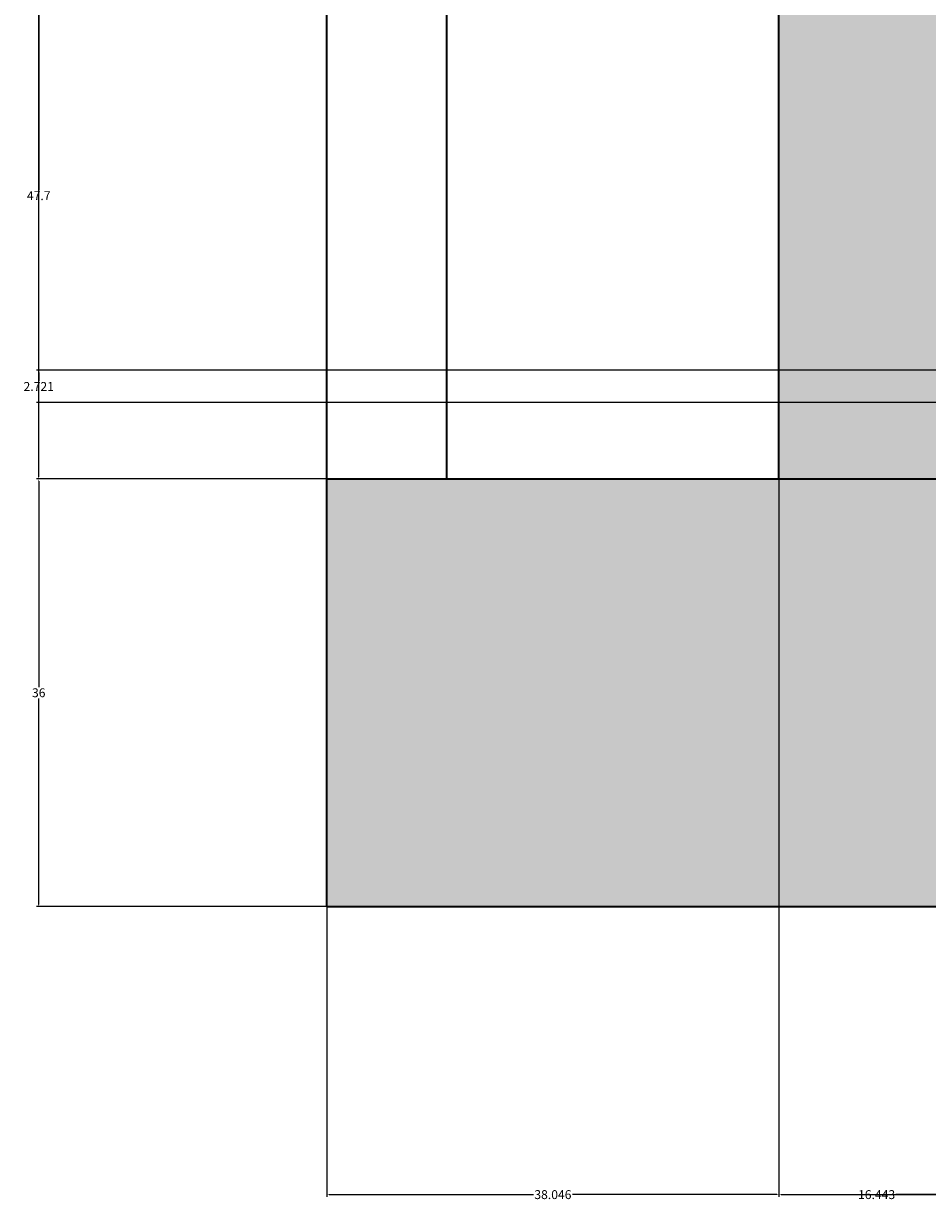
# Model space of a CAD drawing. Units: inches. Extents: x 62 to 566, y 66 to 528.
# Tile 1 of 20: x 62 to 138, y 66 to 165. Entities that reach past the tile are written whole.
import ezdxf

# ---------------------------------------------------------------- set-up
doc = ezdxf.new("R2010")
doc.units = ezdxf.units.IN
doc.header["$MEASUREMENT"] = 0
for name, color, linetype, lineweight in [('A-ANNO-DIMS', 2, 'Continuous', 18), ('A-ELEV', 7, 'Continuous', 35), ('A-WALL-PATT', 8, 'Continuous', 13)]:
    doc.layers.add(name, color=color, linetype=linetype, lineweight=lineweight)
doc.styles.get("Standard").update_dxf_attribs({"font": 'arial.ttf'})
doc.dimstyles.get("Standard").update_dxf_attribs({"dimtxt": 0.75, "dimasz": 0.18, "dimexe": 0.18, "dimexo": 0.0625, "dimgap": 0.09, "dimtad": 0, "dimtih": 1, "dimtoh": 1, "dimdec": 4, "dimzin": 0, "dimdsep": 46, "dimlunit": 4, "dimtxsty": 'Standard', "dimcen": 0.09, "dimadec": 0, "dimazin": 0, "dimtfac": 1, "dimtdec": 4, "dimtofl": 0, "dimtmove": 0, "dimatfit": 3, "dimfxl": 1, "dimtolj": 1, "dimtzin": 0, "dimarcsym": 0})

# ---------------------------------------------------------------- blocks, each defined once
blk = doc.blocks.new('*D7')
at = {"layer": 'A-ANNO-DIMS', "color": 0, "lineweight": -2, "transparency": 16777216}
for p, q in [((125.942, 126.306), (125.942, 65.939)), ((87.896, 90.306), (87.896, 65.939)), ((88.076, 66.119), (105.273, 66.119)), ((125.762, 66.119), (108.565, 66.119))]:
    blk.add_line(p, q, dxfattribs=at)
at = {"layer": 'A-ANNO-DIMS', "color": 0, "transparency": 16777216}
for points in [[(88.076, 66.149), (88.076, 66.089), (87.896, 66.119)], [(125.762, 66.149), (125.762, 66.089), (125.942, 66.119)]]:
    blk.add_solid(points, dxfattribs=at)
at = {"layer": 'Defpoints', "color": 0, "transparency": 16777216}
for p in [(125.942, 126.369), (87.896, 90.369), (125.942, 66.119)]:
    blk.add_point(p, dxfattribs=at)
at = {"layer": 'A-ANNO-DIMS', "color": 0, "transparency": 16777216, "insert": (106.919, 66.119), "char_height": 0.75, "attachment_point": 5}
blk.add_mtext('\\A1;38.046', dxfattribs=at)
blk = doc.blocks.new('*D8')
at = {"layer": 'A-ANNO-DIMS', "color": 0, "lineweight": -2, "transparency": 16777216}
for p, q in [((284.202, 271.35), (284.202, 65.939)), ((125.942, 126.306), (125.942, 65.939)), ((126.122, 66.119), (203.461, 66.119)), ((284.022, 66.119), (206.683, 66.119))]:
    blk.add_line(p, q, dxfattribs=at)
at = {"layer": 'A-ANNO-DIMS', "color": 0, "transparency": 16777216}
for points in [[(126.122, 66.149), (126.122, 66.089), (125.942, 66.119)], [(284.022, 66.149), (284.022, 66.089), (284.202, 66.119)]]:
    blk.add_solid(points, dxfattribs=at)
at = {"layer": 'Defpoints', "color": 0, "transparency": 16777216}
for p in [(284.202, 271.413), (125.942, 126.369), (284.202, 66.119)]:
    blk.add_point(p, dxfattribs=at)
at = {"layer": 'A-ANNO-DIMS', "color": 0, "transparency": 16777216, "insert": (205.072, 66.119), "char_height": 0.75, "attachment_point": 5}
blk.add_mtext('\\A1;158.26', dxfattribs=at)
blk = doc.blocks.new('*D16')
at = {"layer": 'A-ANNO-DIMS', "color": 0, "lineweight": -2, "transparency": 16777216}
for p, q in [((87.834, 126.369), (63.466, 126.369)), ((63.646, 126.189), (63.646, 108.842)), ((63.646, 90.549), (63.646, 107.895)), ((284.14, 90.369), (63.466, 90.369))]:
    blk.add_line(p, q, dxfattribs=at)
at = {"layer": 'A-ANNO-DIMS', "color": 0, "transparency": 16777216}
for points in [[(63.616, 126.189), (63.676, 126.189), (63.646, 126.369)], [(63.616, 90.549), (63.676, 90.549), (63.646, 90.369)]]:
    blk.add_solid(points, dxfattribs=at)
at = {"layer": 'Defpoints', "color": 0, "transparency": 16777216}
for p in [(63.646, 126.369), (87.896, 126.369), (284.202, 90.369)]:
    blk.add_point(p, dxfattribs=at)
at = {"layer": 'A-ANNO-DIMS', "color": 0, "transparency": 16777216, "insert": (63.646, 108.369), "char_height": 0.75, "attachment_point": 5}
blk.add_mtext('\\A1;36', dxfattribs=at)
blk = doc.blocks.new('*D17')
at = {"layer": 'A-ANNO-DIMS', "color": 0, "lineweight": -2, "transparency": 16777216}
for p, q in [((87.833694, 174.065908), (63.466194, 174.065908)), ((63.646194, 173.885908), (63.646194, 150.682257)), ((63.646194, 126.548606), (63.646194, 149.752257)), ((87.833694, 126.368606), (63.466194, 126.368606))]:
    blk.add_line(p, q, dxfattribs=at)
at = {"layer": 'A-ANNO-DIMS', "color": 0, "transparency": 16777216}
for points in [[(63.616194, 173.885908), (63.676194, 173.885908), (63.646194, 174.065908)], [(63.616194, 126.548606), (63.676194, 126.548606), (63.646194, 126.368606)]]:
    blk.add_solid(points, dxfattribs=at)
at = {"layer": 'Defpoints', "color": 0, "transparency": 16777216}
for p in [(63.646194, 174.065908), (87.896194, 174.065908), (87.896194, 126.368606)]:
    blk.add_point(p, dxfattribs=at)
at = {"layer": 'A-ANNO-DIMS', "color": 0, "transparency": 16777216, "insert": (63.646194, 150.217257), "char_height": 0.75, "attachment_point": 5}
blk.add_mtext('\\A1;47.7', dxfattribs=at)
blk = doc.blocks.new('*D35')
at = {"layer": 'A-ANNO-DIMS', "color": 0, "lineweight": -2, "transparency": 16777216}
for p, q in [((125.942, 461.98), (125.942, 65.939)), ((142.385, 445.044), (142.385, 65.939)), ((126.122, 66.119), (132.552, 66.119)), ((142.205, 66.119), (135.775, 66.119))]:
    blk.add_line(p, q, dxfattribs=at)
at = {"layer": 'A-ANNO-DIMS', "color": 0, "transparency": 16777216}
for points in [[(126.122, 66.149), (126.122, 66.089), (125.942, 66.119)], [(142.205, 66.149), (142.205, 66.089), (142.385, 66.119)]]:
    blk.add_solid(points, dxfattribs=at)
at = {"layer": 'Defpoints', "color": 0, "transparency": 16777216}
for p in [(125.942, 462.042), (142.385, 445.106), (142.385, 66.119)]:
    blk.add_point(p, dxfattribs=at)
at = {"layer": 'A-ANNO-DIMS', "color": 0, "transparency": 16777216, "insert": (134.163, 66.119), "char_height": 0.75, "attachment_point": 5}
blk.add_mtext('\\A1;16.443', dxfattribs=at)
blk = doc.blocks.new('*D73')
at = {"layer": 'A-ANNO-DIMS', "color": 0, "lineweight": -2, "transparency": 16777216}
for p, q in [((316.148, 236.662), (63.466, 236.662)), ((63.646, 236.482), (63.646, 181.988)), ((63.646, 126.549), (63.646, 181.042)), ((316.148, 126.369), (63.466, 126.369))]:
    blk.add_line(p, q, dxfattribs=at)
at = {"layer": 'A-ANNO-DIMS', "color": 0, "transparency": 16777216}
for points in [[(63.616, 236.482), (63.676, 236.482), (63.646, 236.662)], [(63.616, 126.549), (63.676, 126.549), (63.646, 126.369)]]:
    blk.add_solid(points, dxfattribs=at)
at = {"layer": 'Defpoints', "color": 0, "transparency": 16777216}
for p in [(63.646, 236.662), (316.21, 236.662), (316.21, 126.369)]:
    blk.add_point(p, dxfattribs=at)
at = {"layer": 'A-ANNO-DIMS', "color": 0, "transparency": 16777216, "insert": (63.646, 181.515), "char_height": 0.75, "attachment_point": 5}
blk.add_mtext('\\A1;110.3', dxfattribs=at)
blk = doc.blocks.new('*D129')
at = {"layer": 'A-ANNO-DIMS', "color": 0, "lineweight": -2, "transparency": 16777216}
for p, q in [((220.527, 135.516), (63.466, 135.516)), ((63.646, 135.336), (63.646, 134.622)), ((220.527, 132.795), (63.466, 132.795)), ((63.646, 132.975), (63.646, 133.689))]:
    blk.add_line(p, q, dxfattribs=at)
at = {"layer": 'A-ANNO-DIMS', "color": 0, "transparency": 16777216}
for points in [[(63.616, 135.336), (63.676, 135.336), (63.646, 135.516)], [(63.616, 132.975), (63.676, 132.975), (63.646, 132.795)]]:
    blk.add_solid(points, dxfattribs=at)
at = {"layer": 'Defpoints', "color": 0, "transparency": 16777216}
for p in [(63.646, 135.516), (220.59, 135.516), (220.59, 132.795)]:
    blk.add_point(p, dxfattribs=at)
at = {"layer": 'A-ANNO-DIMS', "color": 0, "transparency": 16777216, "insert": (63.646, 134.155), "char_height": 0.75, "attachment_point": 5}
blk.add_mtext('\\A1;2.721', dxfattribs=at)

msp = doc.modelspace()

# ---------------------------------------------------------------- hatches: boundary and pattern name
at = {"layer": 'A-WALL-PATT'}
h = msp.add_hatch(color=256, dxfattribs=at)
h.dxf.hatch_style = 1
h.paths.add_polyline_path([(416.0836, 462.0423), (125.9418, 462.0423), (125.9418, 414.3686), (125.9418, 270.3686), (125.9418, 126.3686), (142.3851, 126.3686), (142.3851, 270.3686), (142.3851, 414.3686), (142.3851, 445.1064), (284.2021, 445.1064), (416.0836, 445.1064)])
h.paths.add_polyline_path([(435.3945, 503.0423), (426.3652, 503.0423), (120.4058, 503.0423), (120.4058, 501.0423), (125.9418, 501.0423), (416.0836, 501.0423), (426.3652, 501.0423), (430.6938, 501.0423), (435.3945, 501.0423)])
h.paths.add_polyline_path([(439.6878, 352.4848), (392.4793, 352.4848), (392.4793, 307.4128), (217.2752, 307.4128), (217.2752, 295.4098), (217.2752, 271.4128), (272.0586, 271.4128), (439.6878, 271.4128)])
h.paths.add_polyline_path([(248.0143, 297.1682), (255.6783, 297.1682), (255.6783, 280.0423), (248.0143, 280.0423)], flags=16)
h.paths.add_polyline_path([(235.4641, 280.0423), (227.8001, 280.0423), (227.8001, 297.1682), (235.4641, 297.1682)], flags=16)
h.paths.add_polyline_path([(270.4427, 297.1682), (278.1067, 297.1682), (278.1067, 280.0423), (270.4427, 280.0423)], flags=16)
h.paths.add_polyline_path([(296.3755, 297.1682), (304.0395, 297.1682), (304.0395, 280.0423), (296.3755, 280.0423)], flags=16)
h.paths.add_polyline_path([(319.2543, 297.1682), (326.9183, 297.1682), (326.9183, 280.0423), (319.2543, 280.0423)], flags=16)
h.paths.add_polyline_path([(341.2622, 297.1682), (348.9262, 297.1682), (348.9262, 280.0423), (341.2622, 280.0423)], flags=16)
h.paths.add_polyline_path([(389.2857, 298.3985), (433.8102, 298.3985), (433.8102, 294.9497), (389.2857, 294.9497)], flags=16)
h.paths.add_polyline_path([(389.2857, 291.6038), (433.8102, 291.6038), (433.8102, 288.155), (389.2857, 288.155)], flags=16)
h.paths.add_polyline_path([(389.2857, 284.9607), (433.8102, 284.9607), (433.8102, 281.5119), (389.2857, 281.5119)], flags=16)
h.paths.add_polyline_path([(403.5849, 311.4736), (403.5849, 317.4388), (433.1636, 317.4388), (433.1636, 311.4736)], flags=16)
h.paths.add_polyline_path([(403.5849, 323.1329), (403.5849, 329.0982), (433.1636, 329.0982), (433.1636, 323.1329)], flags=16)
h.paths.add_polyline_path([(403.5849, 334.5211), (403.5849, 340.4863), (433.1636, 340.4863), (433.1636, 334.5211)], flags=16)
h.paths.add_polyline_path([(272.0586, 160.3545), (217.2752, 160.3545), (217.2752, 129.0504), (217.2752, 126.3686), (272.0586, 126.3686)], flags=17)
h.paths.add_polyline_path([(220.5897, 149.5749), (220.5897, 152.296), (267.7931, 152.296), (267.7931, 149.5749)], flags=16)
h.paths.add_polyline_path([(267.7931, 146.6724), (267.7931, 143.9513), (220.5897, 143.9513), (220.5897, 146.6724)], flags=16)
h.paths.add_polyline_path([(220.5897, 155.3799), (220.5897, 158.101), (267.7931, 158.101), (267.7931, 155.3799)], flags=16)
h.paths.add_polyline_path([(267.7931, 140.686), (267.7931, 137.9649), (220.5897, 137.9649), (220.5897, 140.686)], flags=16)
h.paths.add_polyline_path([(267.7931, 135.516), (267.7931, 132.7949), (220.5897, 132.7949), (220.5897, 135.516)], flags=16)
h = msp.add_hatch(dxfattribs=at)
h.set_pattern_fill('ANSI36', color=256, scale=8.8)
h.paths.add_polyline_path([(217.2752, 420.597), (169.0431, 420.597), (169.0431, 126.3686), (217.2752, 126.3686), (217.2752, 129.0504), (217.2752, 271.4128), (217.2752, 295.4128), (217.2752, 307.4128)])
h.paths.add_polyline_path([(282.3509, 501.0423), (125.9418, 501.0423), (125.9418, 465.0423), (282.3509, 465.0423)])
h.paths.add_polyline_path([(209.709, 476.6506), (202.045, 476.6506), (202.045, 493.7764), (209.709, 493.7764)], flags=16)
h.paths.add_polyline_path([(193.9913, 476.6506), (186.3273, 476.6506), (186.3273, 493.7764), (193.9913, 493.7764)], flags=16)
h.paths.add_polyline_path([(177.9243, 476.6506), (170.2603, 476.6506), (170.2603, 493.7764), (177.9243, 493.7764)], flags=16)
h.paths.add_polyline_path([(163.2545, 476.3015), (155.5905, 476.3015), (155.5905, 493.4274), (163.2545, 493.4274)], flags=16)
h.paths.add_polyline_path([(148.2354, 476.3015), (140.5713, 476.3015), (140.5713, 493.4274), (148.2354, 493.4274)], flags=16)
h.paths.add_polyline_path([(284.2021, 126.3686), (87.8962, 126.3686), (87.8962, 114.3686), (87.8962, 90.3686), (284.2021, 90.3686)])
h.paths.add_polyline_path([(474.1214, 126.3686), (396.433, 126.3686), (396.433, 90.3686), (474.1214, 90.3686)])

# ---------------------------------------------------------------- linework, layer by layer
at = {"layer": 'A-ELEV'}
for p, q in [((125.9418, 126.3686), (125.9418, 270.3686)), ((87.8962, 126.3686), (87.8962, 174.0659)), ((97.967, 174.0659), (97.967, 126.3686)), ((87.8962, 114.3686), (87.8962, 126.3686)), ((87.8962, 126.3686), (396.433, 126.3686)), ((87.8962, 90.3686), (87.8962, 114.3686)), ((87.8962, 90.3686), (396.433, 90.3686))]:
    msp.add_line(p, q, dxfattribs=at)

# ---------------------------------------------------------------- dimensions: what is measured, and where the dimension line sits
at = {"layer": 'A-ANNO-DIMS'}
for base, p1, p2, override, picture, middle in [((142.3851, 66.1186), (125.9418, 462.0423), (142.3851, 445.1064), {"dimdec": 3, "dimlfac": 1, "dimrnd": 0, "dimzin": 0, "dimdsep": 46, "dimlunit": 2}, '*D35', (134.1634, 66.1186)), ((284.2021, 66.1186), (125.9418, 126.3686), (284.2021, 271.4128), {"dimdec": 2, "dimlfac": 1, "dimrnd": 0, "dimzin": 0, "dimdsep": 46, "dimlunit": 2}, '*D8', (205.0719, 66.1186)), ((125.9418, 66.1186), (87.8962, 90.3686), (125.9418, 126.3686), {"dimdec": 3, "dimlfac": 1, "dimrnd": 0, "dimzin": 0, "dimdsep": 46, "dimlunit": 2}, '*D7', (106.919, 66.1186))]:
    dim = msp.add_linear_dim(base=base, p1=p1, p2=p2, dimstyle='Standard', override=override, dxfattribs=at)
    dim.commit()
    dim.dimension.update_dxf_attribs({"geometry": picture, "text_midpoint": middle})
for base, p1, p2, override, picture, middle in [((63.6462, 236.6618), (316.2101, 126.3686), (316.2101, 236.6618), {"dimdec": 1, "dimlfac": 1, "dimrnd": 0, "dimzin": 0, "dimdsep": 46, "dimlunit": 2}, '*D73', (63.6462, 181.5152)), ((63.6462, 174.0659), (87.8962, 126.3686), (87.8962, 174.0659), {"dimdec": 1, "dimlfac": 1, "dimrnd": 0, "dimzin": 0, "dimdsep": 46, "dimlunit": 2}, '*D17', (63.6462, 150.2173)), ((63.6462, 135.516), (220.5897, 132.7949), (220.5897, 135.516), {"dimdec": 3, "dimlfac": 1, "dimrnd": 0, "dimzin": 0, "dimdsep": 46, "dimlunit": 2}, '*D129', (63.6462, 134.1554)), ((63.6462, 126.3686), (284.2021, 90.3686), (87.8962, 126.3686), {"dimdec": 0, "dimlfac": 1, "dimrnd": 0, "dimzin": 0, "dimdsep": 46, "dimlunit": 2}, '*D16', (63.6462, 108.3686))]:
    dim = msp.add_linear_dim(base=base, p1=p1, p2=p2, angle=90, dimstyle='Standard', override=override, dxfattribs=at)
    dim.commit()
    dim.dimension.update_dxf_attribs({"geometry": picture, "text_midpoint": middle})

doc.saveas('drawing.dxf')
